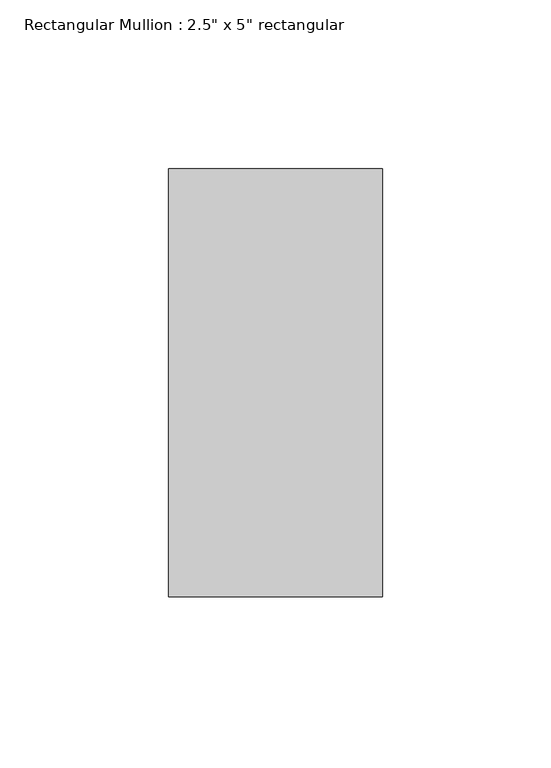
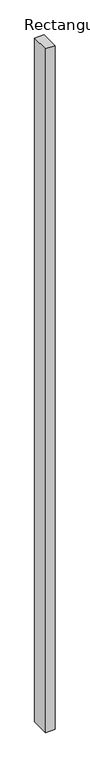
"""IFC4 building model written with IfcOpenShell, lengths in millimetres: member geometry."""

from ifc_helpers import new_model, si_unit, frame, origin, place, context, project, spatial, polyline, outline, extrude, source, transform, mapped, element, save


def member_fc9bce7c(model_context):
    return source(origin(), model_context, "Body", "SweptSolid", [
        extrude(outline(polyline([(0.0, 63.5), (0.0, -63.5), (-63.5, -63.5), (-63.5, 63.5), (0.0, 63.5)])), frame((0.0, 0.0, -4876.8), z_axis=(0.0, 0.0, 1.0), x_axis=(1.0, 0.0, 0.0)), (0.0, 0.0, 1.0), 4876.8),
    ])


if __name__ == "__main__":
    model = new_model("IFC4")
    model_context = context("Model", 3, world=origin())
    ifc_project = project(units=[si_unit("LENGTHUNIT", "METRE", prefix="MILLI")], contexts=[model_context])
    site = spatial("IfcSite", under=ifc_project)
    building = spatial("IfcBuilding", under=site)
    placement = place(None, origin())
    member_shape = member_fc9bce7c(model_context)
    element("IfcMember", 1, ObjectType="Rectangular Mullion : 2.5\" x 5\" rectangular", at=placement, inside=building, context=model_context, shape_type="MappedRepresentation", body=[
        mapped(member_shape, transform((0.0, 0.0, 0.0), x_axis=(1.0, 0.0, 0.0), y_axis=(0.0, 1.0, 0.0), z_axis=(0.0, 0.0, 1.0))),
    ])
    save(model, "model.ifc")

# Revit data of these elements
# Type "Rectangular Mullion : 2.5\" x 5\" rectangular"
#   built-in parameter 1007304 = 0.416667 (stored number, unit not read)
#   built-in parameter 1007301 = 0.104167 (stored number, unit not read)
#   built-in parameter 1007300 = 0.104167 (stored number, unit not read)
# Element 1 (IfcMember, "Rectangular Mullion : 2.5\" x 5\" rectangular")
#   Materials on its faces: "Aluminum"
# Materials
#   "Aluminum": class "Metal", colour RGB 247 247 247, transparency 0, Description = "Aluminum 6061", Cost = 0
